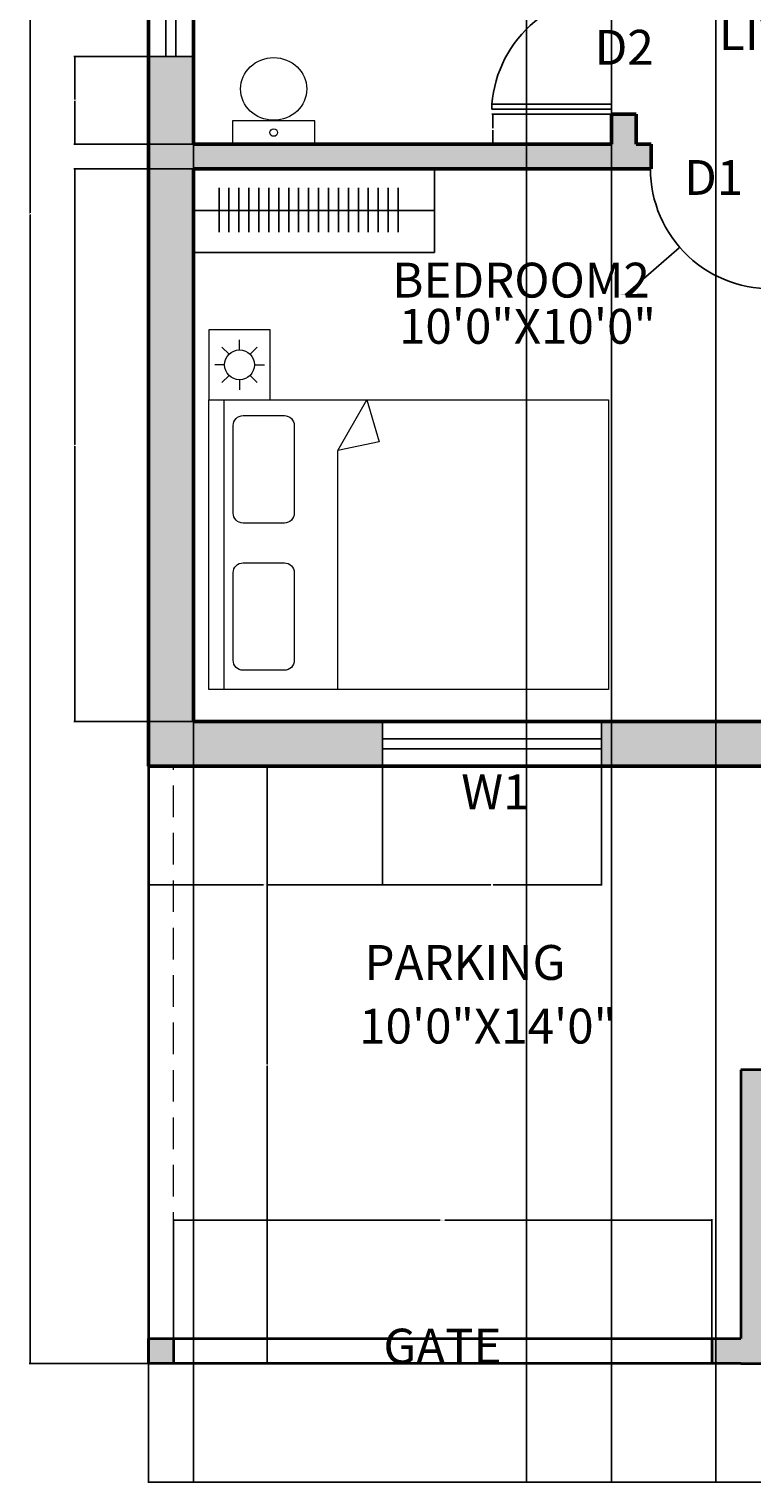
# Model space of a CAD drawing. Units: inches. Extents: x 2715 to 3027, y 1777 to 2287.
# Tile 1 of 4: x 2715 to 2860, y 1777 to 2069. Entities that reach past the tile are written whole.
import ezdxf

# ---------------------------------------------------------------- set-up
doc = ezdxf.new("R2010")
doc.units = ezdxf.units.IN
doc.linetypes.add('DASHED2', pattern=[9.525, 6.35, -3.175])
for name, color, linetype, lineweight in [('A-ANNO-DIMS', 2, 'Continuous', 18), ('A-ANNO-TEXT', 2, 'Continuous', 18), ('A-AREA-IDEN', 2, 'Continuous', 18), ('A-DOOR', 111, 'Continuous', 25), ('A-FLOR-CASE', 201, 'Continuous', 25), ('A-FLOR-FIXT', 201, 'Continuous', 18), ('A-FURN', 201, 'Continuous', 18), ('A-GLAZ', 40, 'Continuous', 25), ('A-WALL', 7, 'Continuous', 50), ('A-WALL-HIDN', 255, 'DASHED2', 18), ('A-WALL-PATT', 252, 'Continuous', 13), ('C-SITE', 7, 'Continuous', 35)]:
    doc.layers.add(name, color=color, linetype=linetype, lineweight=lineweight)
doc.styles.get("Standard").update_dxf_attribs({"font": 'arial.ttf'})
doc.dimstyles.get("Standard").update_dxf_attribs({"dimtxt": 0.18, "dimasz": 0.18, "dimexe": 0.18, "dimexo": 0.0625, "dimgap": 0.09, "dimtad": 0, "dimtih": 1, "dimtoh": 1, "dimdec": 4, "dimzin": 0, "dimdsep": 46, "dimtxsty": 'Standard', "dimcen": 0.09, "dimadec": 0, "dimazin": 0, "dimtfac": 1, "dimtdec": 4, "dimtofl": 0, "dimtmove": 0, "dimatfit": 3, "dimfxl": 1, "dimtolj": 1, "dimtzin": 0, "dimarcsym": 0})

# ---------------------------------------------------------------- blocks, each defined once
blk = doc.blocks.new('DOOR-SWING-24')
for p, q in [((0, 1), (0, 2)), ((0, 2), (24, 2)), ((24, 1), (0, 1)), ((24, 2), (24, 1)), ((24, 0), (24, 1))]:
    blk.add_line(p, q)
blk.add_arc((23.93, 0.14), 24, 83.8472, 175.5509)
blk = doc.blocks.new('WC-CLOSE-COUPLED')
blk.add_lwpolyline([(0, 0), (16.56, 0), (16.56, 4.65), (0, 4.65)], close=True)
blk.add_circle((8.28, 2.33), 0.762)
blk.add_ellipse((8.28, 11.08), major_axis=(6.64, 0), ratio=0.947639)
blk = doc.blocks.new('WARDROBE-RAIL')
for p, q in [((8.37, 48.47), (8.37, 0)), ((3.81, 41.16), (12.71, 41.16)), ((3.81, 39.16), (12.71, 39.16)), ((3.81, 37.16), (12.71, 37.16)), ((3.81, 35.16), (12.71, 35.16)), ((3.81, 33.16), (12.71, 33.16)), ((3.81, 31.16), (12.71, 31.16)), ((3.81, 29.16), (12.71, 29.16)), ((3.81, 27.16), (12.71, 27.16)), ((3.81, 25.16), (12.71, 25.16)), ((3.81, 23.16), (12.71, 23.16)), ((3.81, 21.16), (12.71, 21.16)), ((3.81, 19.16), (12.71, 19.16)), ((3.81, 17.16), (12.71, 17.16)), ((3.81, 15.16), (12.71, 15.16)), ((3.81, 13.16), (12.71, 13.16)), ((3.81, 11.16), (12.71, 11.16)), ((3.81, 9.16), (12.71, 9.16)), ((3.81, 7.16), (12.71, 7.16)), ((3.81, 5.16), (12.71, 5.16))]:
    blk.add_line(p, q)
blk.add_lwpolyline([(16.75, 48.47), (0, 48.47), (0, 0), (16.75, 0)], close=True)
blk = doc.blocks.new('VENT-18')
for p, q in [((0, 18), (9, 18)), ((3.5, 0), (3.5, 18)), ((5.5, 0), (5.5, 18)), ((0, 0), (9, 0))]:
    blk.add_line(p, q)
blk = doc.blocks.new('BED-DOUBLE')
for p, q in [((0, 58.2), (3, 58.2)), ((3, 58.2), (3, 0)), ((25.91, 47.99), (31.76, 58.2)), ((31.76, 58.2), (34.26, 49.78)), ((34.26, 49.78), (25.91, 47.99)), ((25.91, 0), (25.91, 47.99))]:
    blk.add_line(p, q)
blk.add_lwpolyline([(0, 58.2), (80.32, 58.2), (80.32, 0), (0, 0)], close=True)
for points in [[(6.9, 55.02), (15.19, 55.02, -0.414214), (17.19, 53.02), (17.19, 35.44, -0.414214), (15.19, 33.44), (6.9, 33.44, -0.414214), (4.9, 35.44), (4.9, 53.02, -0.414214)], [(6.9, 25.45), (15.19, 25.45, -0.414214), (17.19, 23.45), (17.19, 5.86, -0.414214), (15.19, 3.86), (6.9, 3.86, -0.414214), (4.9, 5.86), (4.9, 23.45, -0.414214)]]:
    blk.add_lwpolyline(points, format="xyb", close=True)
blk = doc.blocks.new('NIGHTSTAND-LAMP')
for p, q in [((6.19, 10.04), (6.19, 12.04)), ((4.07, 9.16), (2.65, 10.57)), ((8.31, 9.16), (9.72, 10.57)), ((3.19, 7.04), (1.19, 7.04)), ((9.19, 7.04), (11.19, 7.04)), ((4.07, 4.92), (2.65, 3.5)), ((6.19, 4.04), (6.19, 2.04)), ((8.31, 4.92), (9.72, 3.5))]:
    blk.add_line(p, q)
blk.add_lwpolyline([(0, 0), (12.37, 0), (12.37, 14.07), (0, 14.07)], close=True)
blk.add_circle((6.19, 7.04), 3)
blk = doc.blocks.new('*D25')
at = {"layer": 'A-ANNO-DIMS', "color": 0, "lineweight": -2, "transparency": 16777216}
for p, q in [((2738.92, 1801.28), (2738.92, 1777.36)), ((3002.92, 1801.28), (3002.92, 1777.36)), ((2739.1, 1777.54), (2870.63, 1777.54)), ((3002.74, 1777.54), (2871.21, 1777.54))]:
    blk.add_line(p, q, dxfattribs=at)
at = {"layer": 'A-ANNO-DIMS', "color": 0, "transparency": 16777216}
for points in [[(2739.1, 1777.57), (2739.1, 1777.51), (2738.92, 1777.54)], [(3002.74, 1777.57), (3002.74, 1777.51), (3002.92, 1777.54)]]:
    blk.add_solid(points, dxfattribs=at)
at = {"layer": 'Defpoints', "color": 0, "transparency": 16777216}
for p in [(2738.92, 1801.34), (3002.92, 1801.34), (3002.92, 1777.54)]:
    blk.add_point(p, dxfattribs=at)
at = {"layer": 'A-ANNO-DIMS', "color": 0, "transparency": 16777216, "insert": (2870.92, 1777.54), "char_height": 0.18, "attachment_point": 5}
blk.add_mtext('\\A1;264', dxfattribs=at)
blk = doc.blocks.new('*D26')
at = {"layer": 'A-ANNO-DIMS', "color": 0, "lineweight": -2, "transparency": 16777216}
for p, q in [((2738.85, 2263.34), (2714.93, 2263.34)), ((2715.11, 2263.16), (2715.11, 2032.52)), ((2715.11, 1801.52), (2715.11, 2032.16)), ((2738.85, 1801.34), (2714.93, 1801.34))]:
    blk.add_line(p, q, dxfattribs=at)
at = {"layer": 'A-ANNO-DIMS', "color": 0, "transparency": 16777216}
for points in [[(2715.08, 2263.16), (2715.14, 2263.16), (2715.11, 2263.34)], [(2715.08, 1801.52), (2715.14, 1801.52), (2715.11, 1801.34)]]:
    blk.add_solid(points, dxfattribs=at)
at = {"layer": 'Defpoints', "color": 0, "transparency": 16777216}
for p in [(2715.11, 2263.34), (2738.92, 2263.34), (2738.92, 1801.34)]:
    blk.add_point(p, dxfattribs=at)
at = {"layer": 'A-ANNO-DIMS', "color": 0, "transparency": 16777216, "insert": (2715.11, 2032.34), "char_height": 0.18, "attachment_point": 5}
blk.add_mtext('\\A1;462', dxfattribs=at)
blk = doc.blocks.new('*D44')
at = {"layer": 'A-ANNO-DIMS', "color": 0, "lineweight": -2, "transparency": 16777216}
for p, q in [((2743.92, 1806.4), (2743.92, 1830.33)), ((2744.1, 1830.15), (2797.55, 1830.15)), ((2851.91, 1830.15), (2798.46, 1830.15)), ((2852.09, 1806.4), (2852.09, 1830.33))]:
    blk.add_line(p, q, dxfattribs=at)
at = {"layer": 'A-ANNO-DIMS', "color": 0, "transparency": 16777216}
for points in [[(2744.1, 1830.18), (2744.1, 1830.12), (2743.92, 1830.15)], [(2851.91, 1830.18), (2851.91, 1830.12), (2852.09, 1830.15)]]:
    blk.add_solid(points, dxfattribs=at)
at = {"layer": 'Defpoints', "color": 0, "transparency": 16777216}
for p in [(2852.09, 1830.15), (2743.92, 1806.34), (2852.09, 1806.34)]:
    blk.add_point(p, dxfattribs=at)
at = {"layer": 'A-ANNO-DIMS', "color": 0, "transparency": 16777216, "insert": (2798, 1830.15), "char_height": 0.18, "attachment_point": 5}
blk.add_mtext('\\A1;108.18', dxfattribs=at)
blk = doc.blocks.new('*D47')
at = {"layer": 'A-ANNO-DIMS', "color": 0, "lineweight": -2, "transparency": 16777216}
for p, q in [((2785.96, 1921.28), (2785.96, 1897.36)), ((2829.96, 1921.28), (2829.96, 1897.36)), ((2786.14, 1897.54), (2807.73, 1897.54)), ((2829.78, 1897.54), (2808.18, 1897.54))]:
    blk.add_line(p, q, dxfattribs=at)
at = {"layer": 'A-ANNO-DIMS', "color": 0, "transparency": 16777216}
for points in [[(2786.14, 1897.57), (2786.14, 1897.51), (2785.96, 1897.54)], [(2829.78, 1897.57), (2829.78, 1897.51), (2829.96, 1897.54)]]:
    blk.add_solid(points, dxfattribs=at)
at = {"layer": 'Defpoints', "color": 0, "transparency": 16777216}
for p in [(2785.96, 1921.34), (2829.96, 1921.34), (2785.96, 1897.54)]:
    blk.add_point(p, dxfattribs=at)
at = {"layer": 'A-ANNO-DIMS', "color": 0, "transparency": 16777216, "insert": (2807.96, 1897.54), "char_height": 0.18, "attachment_point": 5}
blk.add_mtext('\\A1;44', dxfattribs=at)
blk = doc.blocks.new('*D48')
at = {"layer": 'A-ANNO-DIMS', "color": 0, "lineweight": -2, "transparency": 16777216}
for p, q in [((2738.92, 1921.28), (2738.92, 1897.36)), ((2785.96, 1921.28), (2785.96, 1897.36)), ((2739.1, 1897.54), (2762.04, 1897.54)), ((2785.78, 1897.54), (2762.83, 1897.54))]:
    blk.add_line(p, q, dxfattribs=at)
at = {"layer": 'A-ANNO-DIMS', "color": 0, "transparency": 16777216}
for points in [[(2739.1, 1897.57), (2739.1, 1897.51), (2738.92, 1897.54)], [(2785.78, 1897.57), (2785.78, 1897.51), (2785.96, 1897.54)]]:
    blk.add_solid(points, dxfattribs=at)
at = {"layer": 'Defpoints', "color": 0, "transparency": 16777216}
for p in [(2738.92, 1921.34), (2785.96, 1921.34), (2738.92, 1897.54)]:
    blk.add_point(p, dxfattribs=at)
at = {"layer": 'A-ANNO-DIMS', "color": 0, "transparency": 16777216, "insert": (2762.44, 1897.54), "char_height": 0.18, "attachment_point": 5}
blk.add_mtext('\\A1;47.04', dxfattribs=at)
blk = doc.blocks.new('*D49')
at = {"layer": 'A-ANNO-DIMS', "color": 0, "lineweight": -2, "transparency": 16777216}
for p, q in [((2738.98, 1921.34), (2762.9, 1921.34)), ((2762.72, 1921.16), (2762.72, 1861.52)), ((2762.72, 1801.52), (2762.72, 1861.16)), ((2738.98, 1801.34), (2762.9, 1801.34))]:
    blk.add_line(p, q, dxfattribs=at)
at = {"layer": 'A-ANNO-DIMS', "color": 0, "transparency": 16777216}
for points in [[(2762.69, 1921.16), (2762.75, 1921.16), (2762.72, 1921.34)], [(2762.69, 1801.52), (2762.75, 1801.52), (2762.72, 1801.34)]]:
    blk.add_solid(points, dxfattribs=at)
at = {"layer": 'Defpoints', "color": 0, "transparency": 16777216}
for p in [(2738.92, 1921.34), (2738.92, 1801.34), (2762.72, 1801.34)]:
    blk.add_point(p, dxfattribs=at)
at = {"layer": 'A-ANNO-DIMS', "color": 0, "transparency": 16777216, "insert": (2762.72, 1861.34), "char_height": 0.18, "attachment_point": 5}
blk.add_mtext('\\A1;120', dxfattribs=at)
blk = doc.blocks.new('*D55')
at = {"layer": 'A-ANNO-DIMS', "color": 0, "lineweight": -2, "transparency": 16777216}
for p, q in [((2747.92, 2146.28), (2747.92, 1777.36)), ((2852.92, 2146.28), (2852.92, 1777.36)), ((2748.1, 1777.54), (2800.13, 1777.54)), ((2852.74, 1777.54), (2800.7, 1777.54))]:
    blk.add_line(p, q, dxfattribs=at)
at = {"layer": 'A-ANNO-DIMS', "color": 0, "transparency": 16777216}
for points in [[(2748.1, 1777.57), (2748.1, 1777.51), (2747.92, 1777.54)], [(2852.74, 1777.57), (2852.74, 1777.51), (2852.92, 1777.54)]]:
    blk.add_solid(points, dxfattribs=at)
at = {"layer": 'Defpoints', "color": 0, "transparency": 16777216}
for p in [(2747.92, 2146.34), (2852.92, 2146.34), (2852.92, 1777.54)]:
    blk.add_point(p, dxfattribs=at)
at = {"layer": 'A-ANNO-DIMS', "color": 0, "transparency": 16777216, "insert": (2800.42, 1777.54), "char_height": 0.18, "attachment_point": 5}
blk.add_mtext('\\A1;105', dxfattribs=at)
blk = doc.blocks.new('*D56')
at = {"layer": 'A-ANNO-DIMS', "color": 0, "lineweight": -2, "transparency": 16777216}
for p, q in [((2814.87, 2096.28), (2814.87, 1777.36)), ((2831.92, 2096.28), (2831.92, 1777.36)), ((2815.05, 1777.54), (2822.94, 1777.54)), ((2831.74, 1777.54), (2823.85, 1777.54))]:
    blk.add_line(p, q, dxfattribs=at)
at = {"layer": 'A-ANNO-DIMS', "color": 0, "transparency": 16777216}
for points in [[(2815.05, 1777.57), (2815.05, 1777.51), (2814.87, 1777.54)], [(2831.74, 1777.57), (2831.74, 1777.51), (2831.92, 1777.54)]]:
    blk.add_solid(points, dxfattribs=at)
at = {"layer": 'Defpoints', "color": 0, "transparency": 16777216}
for p in [(2814.87, 2096.34), (2831.92, 2096.34), (2831.92, 1777.54)]:
    blk.add_point(p, dxfattribs=at)
at = {"layer": 'A-ANNO-DIMS', "color": 0, "transparency": 16777216, "insert": (2823.39, 1777.54), "char_height": 0.18, "attachment_point": 5}
blk.add_mtext('\\A1;17.048', dxfattribs=at)
blk = doc.blocks.new('*D64')
at = {"layer": 'A-ANNO-DIMS', "color": 0, "lineweight": -2, "transparency": 16777216}
for p, q in [((2747.85, 2041.34), (2723.93, 2041.34)), ((2724.11, 2041.16), (2724.11, 1986.02)), ((2724.11, 1930.52), (2724.11, 1985.66)), ((2747.85, 1930.34), (2723.93, 1930.34))]:
    blk.add_line(p, q, dxfattribs=at)
at = {"layer": 'A-ANNO-DIMS', "color": 0, "transparency": 16777216}
for points in [[(2724.08, 2041.16), (2724.14, 2041.16), (2724.11, 2041.34)], [(2724.08, 1930.52), (2724.14, 1930.52), (2724.11, 1930.34)]]:
    blk.add_solid(points, dxfattribs=at)
at = {"layer": 'Defpoints', "color": 0, "transparency": 16777216}
for p in [(2724.11, 2041.34), (2747.92, 2041.34), (2747.92, 1930.34)]:
    blk.add_point(p, dxfattribs=at)
at = {"layer": 'A-ANNO-DIMS', "color": 0, "transparency": 16777216, "insert": (2724.11, 1985.84), "char_height": 0.18, "attachment_point": 5}
blk.add_mtext('\\A1;111', dxfattribs=at)
blk = doc.blocks.new('*D65')
at = {"layer": 'A-ANNO-DIMS', "color": 0, "lineweight": -2, "transparency": 16777216}
for p, q in [((2831.85, 2052.34), (2807.93, 2052.34)), ((2808.11, 2052.16), (2808.11, 2049.52)), ((2808.11, 2046.52), (2808.11, 2049.16)), ((2831.85, 2046.34), (2807.93, 2046.34))]:
    blk.add_line(p, q, dxfattribs=at)
at = {"layer": 'A-ANNO-DIMS', "color": 0, "transparency": 16777216}
for points in [[(2808.08, 2052.16), (2808.14, 2052.16), (2808.11, 2052.34)], [(2808.08, 2046.52), (2808.14, 2046.52), (2808.11, 2046.34)]]:
    blk.add_solid(points, dxfattribs=at)
at = {"layer": 'Defpoints', "color": 0, "transparency": 16777216}
for p in [(2808.11, 2052.34), (2831.92, 2052.34), (2831.92, 2046.34)]:
    blk.add_point(p, dxfattribs=at)
at = {"layer": 'A-ANNO-DIMS', "color": 0, "transparency": 16777216, "insert": (2808.11, 2049.34), "char_height": 0.18, "attachment_point": 5}
blk.add_mtext('\\A1;6', dxfattribs=at)
blk = doc.blocks.new('*D66')
at = {"layer": 'A-ANNO-DIMS', "color": 0, "lineweight": -2, "transparency": 16777216}
for p, q in [((2747.85, 2063.93), (2723.93, 2063.93)), ((2724.11, 2063.75), (2724.11, 2055.32)), ((2724.11, 2046.52), (2724.11, 2054.95)), ((2747.85, 2046.34), (2723.93, 2046.34))]:
    blk.add_line(p, q, dxfattribs=at)
at = {"layer": 'A-ANNO-DIMS', "color": 0, "transparency": 16777216}
for points in [[(2724.08, 2063.75), (2724.14, 2063.75), (2724.11, 2063.93)], [(2724.08, 2046.52), (2724.14, 2046.52), (2724.11, 2046.34)]]:
    blk.add_solid(points, dxfattribs=at)
at = {"layer": 'Defpoints', "color": 0, "transparency": 16777216}
for p in [(2724.11, 2063.93), (2747.92, 2063.93), (2747.92, 2046.34)]:
    blk.add_point(p, dxfattribs=at)
at = {"layer": 'A-ANNO-DIMS', "color": 0, "transparency": 16777216, "insert": (2724.11, 2055.13), "char_height": 0.18, "attachment_point": 5}
blk.add_mtext('\\A1;17.587', dxfattribs=at)
blk = doc.blocks.new('*D77')
at = {"layer": 'A-ANNO-DIMS', "color": 0, "lineweight": -2, "transparency": 16777216}
for p, q in [((2863.69, 2041.32), (2863.87, 2041.32)), ((2863.78, 2041.23), (2863.78, 2041.41)), ((2834.78, 2016.15), (2845.52, 2025.48)), ((2834.6, 2016.15), (2834.78, 2016.15))]:
    blk.add_line(p, q, dxfattribs=at)
at = {"layer": 'A-ANNO-DIMS', "color": 0, "transparency": 16777216}
blk.add_solid([(2845.5, 2025.5), (2845.54, 2025.45), (2845.66, 2025.59)], dxfattribs=at)
at = {"layer": 'Defpoints', "color": 0, "transparency": 16777216}
for p in [(2863.78, 2041.32), (2845.66, 2025.59)]:
    blk.add_point(p, dxfattribs=at)
at = {"layer": 'A-ANNO-DIMS', "color": 0, "transparency": 16777216, "insert": (2834.11, 2016.15), "char_height": 0.18, "attachment_point": 5}
blk.add_mtext('\\A1;3X R24', dxfattribs=at)

msp = doc.modelspace()

# ---------------------------------------------------------------- hatches: boundary and pattern name
at = {"layer": 'A-WALL-PATT'}
h = msp.add_hatch(color=256, dxfattribs=at)
h.dxf.hatch_style = 1
h.paths.add_polyline_path([(2747.9159, 2063.9272), (2738.9159, 2063.9272), (2738.9159, 1921.3404), (2785.9565, 1921.3404), (2785.9565, 1930.3404), (2747.9159, 1930.3404), (2747.9159, 2041.3404), (2796.3888, 2041.3404), (2839.7837, 2041.3404, -0.02609581), (2839.9159, 2043.8404), (2839.9159, 2046.3404), (2836.9159, 2046.3404), (2836.9159, 2052.3404), (2831.9159, 2052.3404), (2831.9159, 2046.3404), (2747.9159, 2046.3404)])
h = msp.add_hatch(color=256, dxfattribs=at)
h.dxf.hatch_style = 1
h.paths.add_polyline_path([(2872.9159, 2046.3404), (2864.9159, 2046.3404), (2864.9159, 2041.3404), (2867.9159, 2041.3404), (2867.9159, 1930.3404), (2829.9565, 1930.3404), (2829.9565, 1921.3404), (2872.9159, 1921.3404), (2872.9159, 1952.3404), (2903.9159, 1952.3404), (2903.9159, 1921.6914), (2912.9159, 1921.6914), (2912.9159, 1952.3404), (2933.4159, 1952.3404), (2933.4159, 1957.3404), (2872.9159, 1957.3404)])
h = msp.add_hatch(color=256, dxfattribs=at)
h.dxf.hatch_style = 1
h.paths.add_polyline_path([(2862.9159, 1855.3404), (2872.9159, 1855.3404), (2872.9159, 1860.3404), (2857.9159, 1860.3404), (2857.9159, 1806.3404), (2852.094, 1806.3404), (2852.094, 1801.3404), (2857.9159, 1801.3404), (2862.9159, 1801.3404)])
h = msp.add_hatch(color=256, dxfattribs=at)
h.dxf.hatch_style = 1
h.paths.add_polyline_path([(2743.9159, 1806.3404), (2738.9159, 1806.3404), (2738.9159, 1801.3404), (2743.9159, 1801.3404)])

# ---------------------------------------------------------------- linework, layer by layer
at = {"layer": 'A-DOOR'}
msp.add_arc((2863.7837, 2041.3247), 24, 173.983171, 267.927858, dxfattribs=at)
at = {"layer": 'A-GLAZ'}
for p, q in [((2785.9565, 1930.3404), (2785.9565, 1921.3404)), ((2829.9565, 1930.3404), (2829.9565, 1921.3404)), ((2785.9565, 1926.8404), (2829.9565, 1926.8404)), ((2785.9565, 1924.8404), (2829.9565, 1924.8404))]:
    msp.add_line(p, q, dxfattribs=at)
at = {"layer": 'A-WALL'}
for p, q in [((2747.9159, 2046.3404), (2747.9159, 2091.3404)), ((2831.9159, 2046.3404), (2831.9159, 2052.3404)), ((2836.9159, 2052.3404), (2831.9159, 2052.3404)), ((2836.9159, 2046.3404), (2836.9159, 2052.3404)), ((2747.9159, 2046.3404), (2831.9159, 2046.3404)), ((2836.9159, 2046.3404), (2839.9159, 2046.3404)), ((2839.9159, 2046.3404), (2839.9159, 2041.3404)), ((2747.9159, 1930.3404), (2747.9159, 2041.3404)), ((2747.9159, 2041.3404), (2839.9159, 2041.3404)), ((2747.9159, 1930.3404), (2867.9159, 1930.3404)), ((2738.9159, 1921.3404), (2872.9159, 1921.3404))]:
    msp.add_line(p, q, dxfattribs=at)
msp.add_lwpolyline([(2738.9159, 1921.3404), (2738.9159, 2263.3404), (3002.9159, 2263.3404), (3002.9159, 1855.3404), (2903.9159, 1855.3404)], dxfattribs=at)
at = {"layer": 'A-WALL-HIDN'}
msp.add_line((2743.9159, 1806.3404), (2743.9159, 1921.3404), dxfattribs=at)
at = {"layer": 'C-SITE'}
for p, q in [((2738.9159, 1921.3404), (2738.9159, 1801.3404)), ((2872.9159, 1860.3404), (2857.9159, 1860.3404)), ((2857.9159, 1860.3404), (2857.9159, 1806.3404)), ((2738.9159, 1801.3404), (2738.9159, 1806.3404)), ((2738.9159, 1806.3404), (2743.9159, 1806.3404)), ((2743.9159, 1806.3404), (2743.9159, 1801.3404)), ((2743.9159, 1806.3404), (2857.9159, 1806.3404)), ((2852.094, 1806.3404), (2852.094, 1801.3404)), ((2857.9159, 1801.3404), (2738.9159, 1801.3404)), ((2857.9159, 1801.3404), (2862.9159, 1801.3404))]:
    msp.add_line(p, q, dxfattribs=at)

# ---------------------------------------------------------------- block references
at = {"layer": 'A-DOOR'}
msp.add_blockref('DOOR-SWING-24', (2807.916, 2052.34), dxfattribs=at)
at = {"layer": 'A-FLOR-CASE', "rotation": 270.0000000000017}
msp.add_blockref('WARDROBE-RAIL', (2747.9154, 2041.34), dxfattribs=at)
at = {"layer": 'A-FLOR-FIXT'}
msp.add_blockref('WC-CLOSE-COUPLED', (2755.784, 2046.34), dxfattribs=at)
at = {"layer": 'A-FURN'}
for name, p in [('NIGHTSTAND-LAMP', (2751.017, 1994.9621)), ('BED-DOUBLE', (2751.017, 1936.7671))]:
    msp.add_blockref(name, p, dxfattribs=at)
at = {"layer": 'A-GLAZ'}
msp.add_blockref('VENT-18', (2738.916, 2063.9268), dxfattribs=at)

# ---------------------------------------------------------------- texts
at = {"layer": 'A-ANNO-TEXT'}
for tag, p in [('D2', (2828.5677, 2062.2907)), ('D1', (2846.5349, 2036.1389)), ('W1', (2801.7597, 1912.6981)), ('GATE', (2786.1195, 1801.3404))]:
    msp.add_attdef(tag, p, '', height=7, dxfattribs=at)
at = {"layer": 'A-AREA-IDEN'}
for tag, p in [('LIVING/DINING', (2853.5433, 2065.2489)), ('BEDROOM2', (2787.8815, 2015.5072)), ('10\'0"X10\'0"', (2789.2446, 2006.2275)), ('PARKING', (2782.3074, 1878.424)), ('10\'0"X14\'0"', (2781.2407, 1865.6345))]:
    msp.add_attdef(tag, p, '', height=7, dxfattribs=at)

# ---------------------------------------------------------------- dimensions: what is measured, and where the dimension line sits
at = {"layer": 'A-ANNO-DIMS'}
for base, p1, p2, angle, override, picture, middle in [((2715.1109, 2263.3404), (2738.9159, 1801.3404), (2738.9159, 2263.3404), 90, {"dimdec": 0, "dimlfac": 1, "dimrnd": 0, "dimzin": 0, "dimdsep": 46, "dimlunit": 2}, '*D26', (2715.1109, 2032.3404)), ((2724.1109, 2063.9272), (2747.9159, 2046.3404), (2747.9159, 2063.9272), 90, {"dimdec": 3, "dimlfac": 1, "dimrnd": 0, "dimzin": 0, "dimdsep": 46, "dimlunit": 2}, '*D66', (2724.1109, 2055.1338)), ((2808.1109, 2052.3404), (2831.9159, 2046.3404), (2831.9159, 2052.3404), 90, {"dimdec": 0, "dimlfac": 1, "dimrnd": 0, "dimzin": 0, "dimdsep": 46, "dimlunit": 2}, '*D65', (2808.1109, 2049.3404)), ((2724.1109, 2041.3404), (2747.9159, 1930.3404), (2747.9159, 2041.3404), 90, {"dimdec": 0, "dimlfac": 1, "dimrnd": 0, "dimzin": 0, "dimdsep": 46, "dimlunit": 2}, '*D64', (2724.1109, 1985.8404)), ((2738.9159, 1897.5354), (2785.9565, 1921.3404), (2738.9159, 1921.3404), 180, {"dimdec": 2, "dimlfac": 1, "dimrnd": 0, "dimzin": 0, "dimdsep": 46, "dimlunit": 2}, '*D48', (2762.4362, 1897.5354)), ((2762.7209, 1801.3404), (2738.9159, 1921.3404), (2738.9159, 1801.3404), 270, {"dimdec": 0, "dimlfac": 1, "dimrnd": 0, "dimzin": 0, "dimdsep": 46, "dimlunit": 2}, '*D49', (2762.7209, 1861.3404)), ((2785.9565, 1897.5354), (2829.9565, 1921.3404), (2785.9565, 1921.3404), 180, {"dimdec": 0, "dimlfac": 1, "dimrnd": 0, "dimzin": 0, "dimdsep": 46, "dimlunit": 2}, '*D47', (2807.9565, 1897.5354))]:
    dim = msp.add_linear_dim(base=base, p1=p1, p2=p2, angle=angle, dimstyle='Standard', override=override, dxfattribs=at)
    dim.commit()
    dim.dimension.update_dxf_attribs({"geometry": picture, "text_midpoint": middle})
for base, p1, p2, override, picture, middle in [((2852.9159, 1777.5354), (2747.9159, 2146.3404), (2852.9159, 2146.3404), {"dimdec": 0, "dimlfac": 1, "dimrnd": 0, "dimzin": 0, "dimdsep": 46, "dimlunit": 2}, '*D55', (2800.4159, 1777.5354)), ((2831.9159, 1777.5354), (2814.8679, 2096.3404), (2831.9159, 2096.3404), {"dimdec": 3, "dimlfac": 1, "dimrnd": 0, "dimzin": 0, "dimdsep": 46, "dimlunit": 2}, '*D56', (2823.3919, 1777.5354)), ((2852.094, 1830.1454), (2743.9159, 1806.3404), (2852.094, 1806.3404), {"dimdec": 2, "dimlfac": 1, "dimrnd": 0, "dimzin": 0, "dimdsep": 46, "dimlunit": 2}, '*D44', (2798.005, 1830.1454)), ((3002.9159, 1777.5354), (2738.9159, 1801.3404), (3002.9159, 1801.3404), {"dimdec": 0, "dimlfac": 1, "dimrnd": 0, "dimzin": 0, "dimdsep": 46, "dimlunit": 2}, '*D25', (2870.9159, 1777.5354))]:
    dim = msp.add_linear_dim(base=base, p1=p1, p2=p2, dimstyle='Standard', override=override, dxfattribs=at)
    dim.commit()
    dim.dimension.update_dxf_attribs({"geometry": picture, "text_midpoint": middle})
dim = msp.add_radius_dim(center=(2863.7837, 2041.3247), mpoint=(2845.6584, 2025.5934), text='3X <>', dimstyle='Standard', override={"dimdec": 0, "dimlfac": 1, "dimrnd": 0, "dimzin": 0, "dimdsep": 46, "dimlunit": 2}, dxfattribs=at)
dim.commit()
dim.dimension.update_dxf_attribs({"geometry": '*D77', "text_midpoint": (2834.1053, 2016.1546), "dimtype": 164})

doc.saveas('drawing.dxf')
